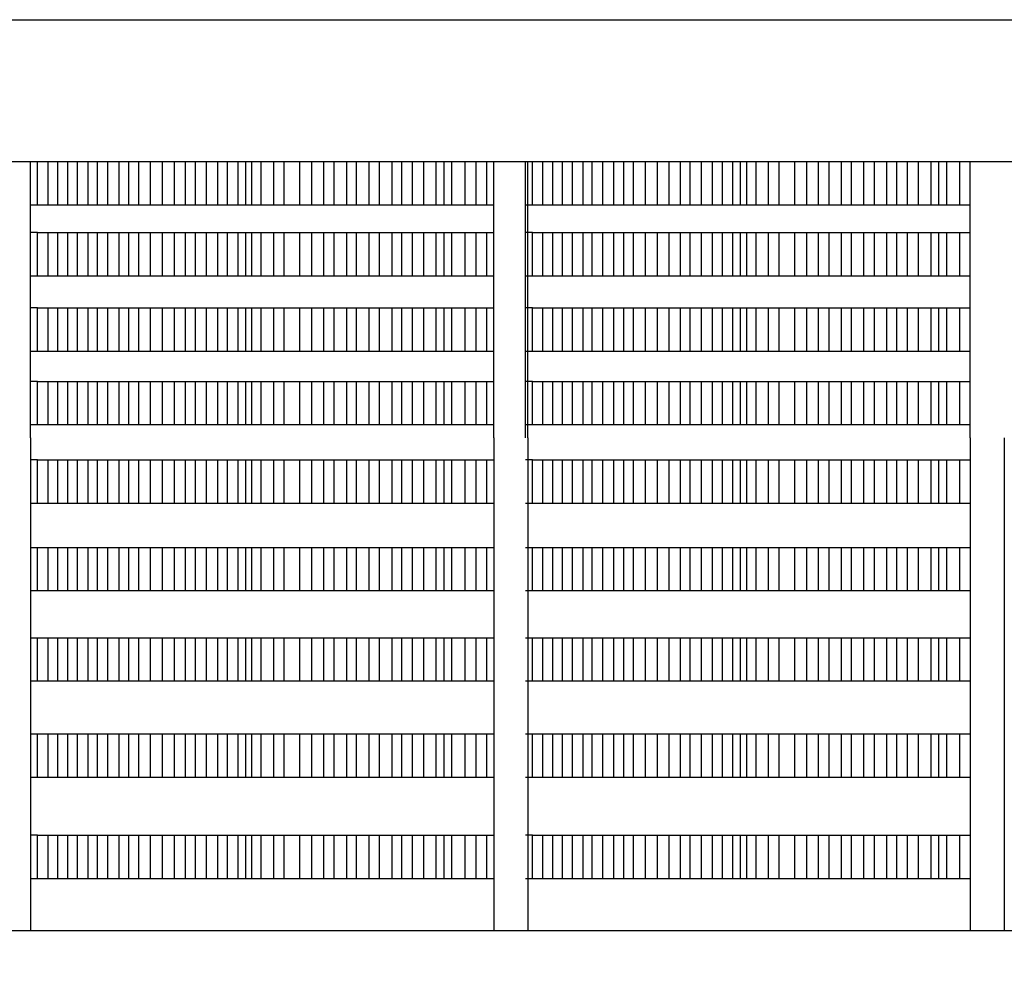
# Model space of a CAD drawing. Units: inches. Extents: x -117 to 121, y -77 to 40.
# Tile 33 of 45: x 34.28 to 45.7, y 10.29 to 21.31. Entities that reach past the tile are written whole.
import ezdxf

# ---------------------------------------------------------------- set-up
doc = ezdxf.new("R2010")
doc.units = ezdxf.units.IN
doc.header["$MEASUREMENT"] = 0
doc.layers.add('A-ANNO-DIMS', color=2, linetype='Continuous', lineweight=18)
doc.layers.add('A-ELEV', color=7, linetype='Continuous', lineweight=25)
doc.styles.get("Standard").update_dxf_attribs({"font": 'arial.ttf'})
doc.dimstyles.get("Standard").update_dxf_attribs({"dimtxt": 0.18, "dimasz": 0.18, "dimexe": 0.18, "dimexo": 0.0625, "dimgap": 0.09, "dimtad": 0, "dimtih": 1, "dimtoh": 1, "dimdec": 4, "dimzin": 0, "dimdsep": 46, "dimtxsty": 'Standard', "dimcen": 0.09, "dimadec": 0, "dimazin": 0, "dimtfac": 1, "dimtdec": 4, "dimtofl": 0, "dimtmove": 0, "dimatfit": 3, "dimfxl": 1, "dimtolj": 1, "dimtzin": 0, "dimarcsym": 0})

# ---------------------------------------------------------------- blocks, each defined once
blk = doc.blocks.new('*D53')
at = {"layer": 'A-ANNO-DIMS', "color": 0, "lineweight": -2, "transparency": 16777216}
for p, q in [((51.69, 10.9), (51.69, -77.193)), ((27.974, 10.841), (27.974, -77.193)), ((28.154, -77.013), (39.367, -77.013)), ((51.51, -77.013), (40.297, -77.013))]:
    blk.add_line(p, q, dxfattribs=at)
at = {"layer": 'A-ANNO-DIMS', "color": 0, "transparency": 16777216}
for points in [[(28.154, -76.983), (28.154, -77.043), (27.974, -77.013)], [(51.51, -76.983), (51.51, -77.043), (51.69, -77.013)]]:
    blk.add_solid(points, dxfattribs=at)
at = {"layer": 'Defpoints', "color": 0, "transparency": 16777216}
for p in [(51.69, 10.962), (27.974, 10.903), (51.69, -77.013)]:
    blk.add_point(p, dxfattribs=at)
at = {"layer": 'A-ANNO-DIMS', "color": 0, "transparency": 16777216, "insert": (39.832, -77.013), "char_height": 0.18, "attachment_point": 5}
blk.add_mtext('\\A1;23.716', dxfattribs=at)

msp = doc.modelspace()

# ---------------------------------------------------------------- linework, layer by layer
at = {"layer": 'A-ELEV'}
for p, q in [((32.0351, 21.3104), (70.6115, 21.3104)), ((27.8529, 19.6653), (51.6089, 19.6653)), ((34.4079, 16.4655), (34.4079, 19.6653)), ((34.4891, 19.1644), (34.4891, 19.6653)), ((34.6111, 19.1644), (34.6111, 19.6653)), ((34.7255, 19.1644), (34.7255, 19.6653)), ((34.8399, 19.1644), (34.8399, 19.6653)), ((34.9543, 19.1644), (34.9543, 19.6653)), ((35.0763, 19.1644), (35.0763, 19.6653)), ((35.1831, 19.1644), (35.1831, 19.6653)), ((35.3051, 19.1644), (35.3051, 19.6653)), ((35.4347, 19.1644), (35.4347, 19.6653)), ((35.5491, 19.1644), (35.5491, 19.6653)), ((35.6635, 19.1644), (35.6635, 19.6653)), ((35.8008, 19.1644), (35.8008, 19.6653)), ((35.9381, 19.1644), (35.9381, 19.6653)), ((36.0753, 19.1644), (36.0753, 19.6653)), ((36.205, 19.1644), (36.205, 19.6653)), ((36.3194, 19.1644), (36.3194, 19.6653)), ((36.449, 19.1644), (36.449, 19.6653)), ((36.5787, 19.1644), (36.5787, 19.6653)), ((36.6931, 19.1644), (36.6931, 19.6653)), ((36.8151, 19.1644), (36.8151, 19.6653)), ((36.9029, 19.1644), (36.9029, 19.6562)), ((36.9752, 19.1644), (36.9752, 19.6653)), ((37.082, 19.1644), (37.082, 19.6653)), ((37.2269, 19.1644), (37.2269, 19.6653)), ((37.3489, 19.1644), (37.3489, 19.6653)), ((37.5319, 19.1644), (37.5319, 19.6653)), ((37.6692, 19.1644), (37.6692, 19.6653)), ((37.8065, 19.1644), (37.8065, 19.6653)), ((37.9285, 19.1644), (37.9285, 19.6653)), ((38.0734, 19.1644), (38.0734, 19.6653)), ((38.1878, 19.1644), (38.1878, 19.6653)), ((38.3327, 19.1644), (38.3327, 19.6653)), ((38.4547, 19.1644), (38.4547, 19.6653)), ((38.5996, 19.1644), (38.5996, 19.6653)), ((38.714, 19.1644), (38.714, 19.6653)), ((38.836, 19.1644), (38.836, 19.6653)), ((38.9657, 19.1644), (38.9657, 19.6653)), ((39.1106, 19.1644), (39.1106, 19.6653)), ((39.2021, 19.1644), (39.2021, 19.6653)), ((39.2936, 19.1644), (39.2936, 19.6653)), ((39.4461, 19.1644), (39.4461, 19.6653)), ((39.5758, 19.1644), (39.5758, 19.6653)), ((39.6978, 19.1644), (39.6978, 19.6653)), ((39.7801, 16.4655), (39.7801, 19.6653)), ((40.1443, 16.4655), (40.1443, 19.6653)), ((40.1744, 16.4655), (40.1744, 19.6653)), ((40.2255, 19.1644), (40.2255, 19.6653)), ((40.3475, 19.1644), (40.3475, 19.6653)), ((40.4619, 19.1644), (40.4619, 19.6653)), ((40.5763, 19.1644), (40.5763, 19.6653)), ((40.6907, 19.1644), (40.6907, 19.6653)), ((40.8127, 19.1644), (40.8127, 19.6653)), ((40.9194, 19.1644), (40.9194, 19.6653)), ((41.0415, 19.1644), (41.0415, 19.6653)), ((41.1711, 19.1644), (41.1711, 19.6653)), ((41.2855, 19.1644), (41.2855, 19.6653)), ((41.3999, 19.1644), (41.3999, 19.6653)), ((41.5372, 19.1644), (41.5372, 19.6653)), ((41.6744, 19.1644), (41.6744, 19.6653)), ((41.8117, 19.1644), (41.8117, 19.6653)), ((41.9414, 19.1644), (41.9414, 19.6653)), ((42.0557, 19.1644), (42.0557, 19.6653)), ((42.1854, 19.1644), (42.1854, 19.6653)), ((42.315, 19.1644), (42.315, 19.6653)), ((42.4294, 19.1644), (42.4294, 19.6653)), ((42.5514, 19.1644), (42.5514, 19.6653)), ((42.6392, 19.1644), (42.6392, 19.6562)), ((42.7116, 19.1644), (42.7116, 19.6653)), ((42.8184, 19.1644), (42.8184, 19.6653)), ((42.9633, 19.1644), (42.9633, 19.6653)), ((43.0853, 19.1644), (43.0853, 19.6653)), ((43.2683, 19.1644), (43.2683, 19.6653)), ((43.4056, 19.1644), (43.4056, 19.6653)), ((43.5429, 19.1644), (43.5429, 19.6653)), ((43.6649, 19.1644), (43.6649, 19.6653)), ((43.8098, 19.1644), (43.8098, 19.6653)), ((43.9242, 19.1644), (43.9242, 19.6653)), ((44.0691, 19.1644), (44.0691, 19.6653)), ((44.1911, 19.1644), (44.1911, 19.6653)), ((44.336, 19.1644), (44.336, 19.6653)), ((44.4504, 19.1644), (44.4504, 19.6653)), ((44.5724, 19.1644), (44.5724, 19.6653)), ((44.702, 19.1644), (44.702, 19.6653)), ((44.8469, 19.1644), (44.8469, 19.6653)), ((44.9384, 19.1644), (44.9384, 19.6653)), ((45.03, 19.1644), (45.03, 19.6653)), ((45.1825, 19.1644), (45.1825, 19.6653)), ((45.3002, 16.4655), (45.3002, 19.6653)), ((34.4079, 19.1644), (39.7801, 19.1644)), ((40.1443, 19.1644), (45.3002, 19.1644)), ((34.4891, 18.8424), (34.4079, 18.8424)), ((34.4891, 18.3415), (34.4891, 18.8424)), ((34.4891, 18.8424), (39.7801, 18.8424)), ((34.6111, 18.3415), (34.6111, 18.8424)), ((34.7255, 18.3415), (34.7255, 18.8424)), ((34.8399, 18.3415), (34.8399, 18.8424)), ((34.9543, 18.3415), (34.9543, 18.8424)), ((35.0763, 18.3415), (35.0763, 18.8424)), ((35.1831, 18.3415), (35.1831, 18.8424)), ((35.3051, 18.3415), (35.3051, 18.8424)), ((35.4347, 18.3415), (35.4347, 18.8424)), ((35.5491, 18.3415), (35.5491, 18.8424)), ((35.6635, 18.3415), (35.6635, 18.8424)), ((35.8008, 18.3415), (35.8008, 18.8424)), ((35.9381, 18.3415), (35.9381, 18.8424)), ((36.0753, 18.3415), (36.0753, 18.8424)), ((36.205, 18.3415), (36.205, 18.8424)), ((36.3194, 18.3415), (36.3194, 18.8424)), ((36.449, 18.3415), (36.449, 18.8424)), ((36.5787, 18.3415), (36.5787, 18.8424)), ((36.6931, 18.3415), (36.6931, 18.8424)), ((36.8151, 18.3415), (36.8151, 18.8424)), ((36.9029, 18.3415), (36.9029, 18.8333)), ((36.9752, 18.3415), (36.9752, 18.8424)), ((37.082, 18.3415), (37.082, 18.8424)), ((37.2269, 18.3415), (37.2269, 18.8424)), ((37.3489, 18.3415), (37.3489, 18.8424)), ((37.5319, 18.3415), (37.5319, 18.8424)), ((37.6692, 18.3415), (37.6692, 18.8424)), ((37.8065, 18.3415), (37.8065, 18.8424)), ((37.9285, 18.3415), (37.9285, 18.8424)), ((38.0734, 18.3415), (38.0734, 18.8424)), ((38.1878, 18.3415), (38.1878, 18.8424)), ((38.3327, 18.3415), (38.3327, 18.8424)), ((38.4547, 18.3415), (38.4547, 18.8424)), ((38.5996, 18.3415), (38.5996, 18.8424)), ((38.714, 18.3415), (38.714, 18.8424)), ((38.836, 18.3415), (38.836, 18.8424)), ((38.9657, 18.3415), (38.9657, 18.8424)), ((39.1106, 18.3415), (39.1106, 18.8424)), ((39.2021, 18.3415), (39.2021, 18.8424)), ((39.2936, 18.3415), (39.2936, 18.8424)), ((39.4461, 18.3415), (39.4461, 18.8424)), ((39.5758, 18.3415), (39.5758, 18.8424)), ((39.6978, 18.3415), (39.6978, 18.8424)), ((40.2255, 18.8424), (40.1443, 18.8424)), ((40.2255, 18.3415), (40.2255, 18.8424)), ((40.2255, 18.8424), (45.3002, 18.8424)), ((40.3475, 18.3415), (40.3475, 18.8424)), ((40.4619, 18.3415), (40.4619, 18.8424)), ((40.5763, 18.3415), (40.5763, 18.8424)), ((40.6907, 18.3415), (40.6907, 18.8424)), ((40.8127, 18.3415), (40.8127, 18.8424)), ((40.9194, 18.3415), (40.9194, 18.8424)), ((41.0415, 18.3415), (41.0415, 18.8424)), ((41.1711, 18.3415), (41.1711, 18.8424)), ((41.2855, 18.3415), (41.2855, 18.8424)), ((41.3999, 18.3415), (41.3999, 18.8424)), ((41.5372, 18.3415), (41.5372, 18.8424)), ((41.6744, 18.3415), (41.6744, 18.8424)), ((41.8117, 18.3415), (41.8117, 18.8424)), ((41.9414, 18.3415), (41.9414, 18.8424)), ((42.0557, 18.3415), (42.0557, 18.8424)), ((42.1854, 18.3415), (42.1854, 18.8424)), ((42.315, 18.3415), (42.315, 18.8424)), ((42.4294, 18.3415), (42.4294, 18.8424)), ((42.5514, 18.3415), (42.5514, 18.8424)), ((42.6392, 18.3415), (42.6392, 18.8333)), ((42.7116, 18.3415), (42.7116, 18.8424)), ((42.8184, 18.3415), (42.8184, 18.8424)), ((42.9633, 18.3415), (42.9633, 18.8424)), ((43.0853, 18.3415), (43.0853, 18.8424)), ((43.2683, 18.3415), (43.2683, 18.8424)), ((43.4056, 18.3415), (43.4056, 18.8424)), ((43.5429, 18.3415), (43.5429, 18.8424)), ((43.6649, 18.3415), (43.6649, 18.8424)), ((43.8098, 18.3415), (43.8098, 18.8424)), ((43.9242, 18.3415), (43.9242, 18.8424)), ((44.0691, 18.3415), (44.0691, 18.8424)), ((44.1911, 18.3415), (44.1911, 18.8424)), ((44.336, 18.3415), (44.336, 18.8424)), ((44.4504, 18.3415), (44.4504, 18.8424)), ((44.5724, 18.3415), (44.5724, 18.8424)), ((44.702, 18.3415), (44.702, 18.8424)), ((44.8469, 18.3415), (44.8469, 18.8424)), ((44.9384, 18.3415), (44.9384, 18.8424)), ((45.03, 18.3415), (45.03, 18.8424)), ((45.1825, 18.3415), (45.1825, 18.8424)), ((34.4079, 18.3415), (39.7801, 18.3415)), ((40.1443, 18.3415), (45.3002, 18.3415)), ((34.4891, 17.9696), (34.4079, 17.9696)), ((34.4891, 17.4687), (34.4891, 17.9696)), ((34.4891, 17.9696), (39.7801, 17.9696)), ((34.6111, 17.4687), (34.6111, 17.9696)), ((34.7255, 17.4687), (34.7255, 17.9696)), ((34.8399, 17.4687), (34.8399, 17.9696)), ((34.9543, 17.4687), (34.9543, 17.9696)), ((35.0763, 17.4687), (35.0763, 17.9696)), ((35.1831, 17.4687), (35.1831, 17.9696)), ((35.3051, 17.4687), (35.3051, 17.9696)), ((35.4347, 17.4687), (35.4347, 17.9696)), ((35.5491, 17.4687), (35.5491, 17.9696)), ((35.6635, 17.4687), (35.6635, 17.9696)), ((35.8008, 17.4687), (35.8008, 17.9696)), ((35.9381, 17.4687), (35.9381, 17.9696)), ((36.0753, 17.4687), (36.0753, 17.9696)), ((36.205, 17.4687), (36.205, 17.9696)), ((36.3194, 17.4687), (36.3194, 17.9696)), ((36.449, 17.4687), (36.449, 17.9696)), ((36.5787, 17.4687), (36.5787, 17.9696)), ((36.6931, 17.4687), (36.6931, 17.9696)), ((36.8151, 17.4687), (36.8151, 17.9696)), ((36.9029, 17.4687), (36.9029, 17.9605)), ((36.9752, 17.4687), (36.9752, 17.9696)), ((37.082, 17.4687), (37.082, 17.9696)), ((37.2269, 17.4687), (37.2269, 17.9696)), ((37.3489, 17.4687), (37.3489, 17.9696)), ((37.5319, 17.4687), (37.5319, 17.9696)), ((37.6692, 17.4687), (37.6692, 17.9696)), ((37.8065, 17.4687), (37.8065, 17.9696)), ((37.9285, 17.4687), (37.9285, 17.9696)), ((38.0734, 17.4687), (38.0734, 17.9696)), ((38.1878, 17.4687), (38.1878, 17.9696)), ((38.3327, 17.4687), (38.3327, 17.9696)), ((38.4547, 17.4687), (38.4547, 17.9696)), ((38.5996, 17.4687), (38.5996, 17.9696)), ((38.714, 17.4687), (38.714, 17.9696)), ((38.836, 17.4687), (38.836, 17.9696)), ((38.9657, 17.4687), (38.9657, 17.9696)), ((39.1106, 17.4687), (39.1106, 17.9696)), ((39.2021, 17.4687), (39.2021, 17.9696)), ((39.2936, 17.4687), (39.2936, 17.9696)), ((39.4461, 17.4687), (39.4461, 17.9696)), ((39.5758, 17.4687), (39.5758, 17.9696)), ((39.6978, 17.4687), (39.6978, 17.9696)), ((40.2255, 17.9696), (40.1443, 17.9696)), ((40.2255, 17.4687), (40.2255, 17.9696)), ((40.2255, 17.9696), (45.3002, 17.9696)), ((40.3475, 17.4687), (40.3475, 17.9696)), ((40.4619, 17.4687), (40.4619, 17.9696)), ((40.5763, 17.4687), (40.5763, 17.9696)), ((40.6907, 17.4687), (40.6907, 17.9696)), ((40.8127, 17.4687), (40.8127, 17.9696)), ((40.9194, 17.4687), (40.9194, 17.9696)), ((41.0415, 17.4687), (41.0415, 17.9696)), ((41.1711, 17.4687), (41.1711, 17.9696)), ((41.2855, 17.4687), (41.2855, 17.9696)), ((41.3999, 17.4687), (41.3999, 17.9696)), ((41.5372, 17.4687), (41.5372, 17.9696)), ((41.6744, 17.4687), (41.6744, 17.9696)), ((41.8117, 17.4687), (41.8117, 17.9696)), ((41.9414, 17.4687), (41.9414, 17.9696)), ((42.0557, 17.4687), (42.0557, 17.9696)), ((42.1854, 17.4687), (42.1854, 17.9696)), ((42.315, 17.4687), (42.315, 17.9696)), ((42.4294, 17.4687), (42.4294, 17.9696)), ((42.5514, 17.4687), (42.5514, 17.9696)), ((42.6392, 17.4687), (42.6392, 17.9605)), ((42.7116, 17.4687), (42.7116, 17.9696)), ((42.8184, 17.4687), (42.8184, 17.9696)), ((42.9633, 17.4687), (42.9633, 17.9696)), ((43.0853, 17.4687), (43.0853, 17.9696)), ((43.2683, 17.4687), (43.2683, 17.9696)), ((43.4056, 17.4687), (43.4056, 17.9696)), ((43.5429, 17.4687), (43.5429, 17.9696)), ((43.6649, 17.4687), (43.6649, 17.9696)), ((43.8098, 17.4687), (43.8098, 17.9696)), ((43.9242, 17.4687), (43.9242, 17.9696)), ((44.0691, 17.4687), (44.0691, 17.9696)), ((44.1911, 17.4687), (44.1911, 17.9696)), ((44.336, 17.4687), (44.336, 17.9696)), ((44.4504, 17.4687), (44.4504, 17.9696)), ((44.5724, 17.4687), (44.5724, 17.9696)), ((44.702, 17.4687), (44.702, 17.9696)), ((44.8469, 17.4687), (44.8469, 17.9696)), ((44.9384, 17.4687), (44.9384, 17.9696)), ((45.03, 17.4687), (45.03, 17.9696)), ((45.1825, 17.4687), (45.1825, 17.9696)), ((34.4079, 17.4687), (39.7801, 17.4687)), ((40.1443, 17.4687), (45.3002, 17.4687)), ((34.4891, 17.1187), (34.4079, 17.1187)), ((34.4891, 16.6179), (34.4891, 17.1187)), ((34.4891, 17.1187), (39.7801, 17.1187)), ((34.6111, 16.6179), (34.6111, 17.1187)), ((34.7255, 16.6179), (34.7255, 17.1187)), ((34.8399, 16.6179), (34.8399, 17.1187)), ((34.9543, 16.6179), (34.9543, 17.1187)), ((35.0763, 16.6179), (35.0763, 17.1187)), ((35.1831, 16.6179), (35.1831, 17.1187)), ((35.3051, 16.6179), (35.3051, 17.1187)), ((35.4347, 16.6179), (35.4347, 17.1187)), ((35.5491, 16.6179), (35.5491, 17.1187)), ((35.6635, 16.6179), (35.6635, 17.1187)), ((35.8008, 16.6179), (35.8008, 17.1187)), ((35.9381, 16.6179), (35.9381, 17.1187)), ((36.0753, 16.6179), (36.0753, 17.1187)), ((36.205, 16.6179), (36.205, 17.1187)), ((36.3194, 16.6179), (36.3194, 17.1187)), ((36.449, 16.6179), (36.449, 17.1187)), ((36.5787, 16.6179), (36.5787, 17.1187)), ((36.6931, 16.6179), (36.6931, 17.1187)), ((36.8151, 16.6179), (36.8151, 17.1187)), ((36.9029, 16.6179), (36.9029, 17.1097)), ((36.9752, 16.6179), (36.9752, 17.1187)), ((37.082, 16.6179), (37.082, 17.1187)), ((37.2269, 16.6179), (37.2269, 17.1187)), ((37.3489, 16.6179), (37.3489, 17.1187)), ((37.5319, 16.6179), (37.5319, 17.1187)), ((37.6692, 16.6179), (37.6692, 17.1187)), ((37.8065, 16.6179), (37.8065, 17.1187)), ((37.9285, 16.6179), (37.9285, 17.1187)), ((38.0734, 16.6179), (38.0734, 17.1187)), ((38.1878, 16.6179), (38.1878, 17.1187)), ((38.3327, 16.6179), (38.3327, 17.1187)), ((38.4547, 16.6179), (38.4547, 17.1187)), ((38.5996, 16.6179), (38.5996, 17.1187)), ((38.714, 16.6179), (38.714, 17.1187)), ((38.836, 16.6179), (38.836, 17.1187)), ((38.9657, 16.6179), (38.9657, 17.1187)), ((39.1106, 16.6179), (39.1106, 17.1187)), ((39.2021, 16.6179), (39.2021, 17.1187)), ((39.2936, 16.6179), (39.2936, 17.1187)), ((39.4461, 16.6179), (39.4461, 17.1187)), ((39.5758, 16.6179), (39.5758, 17.1187)), ((39.6978, 16.6179), (39.6978, 17.1187)), ((40.2255, 17.1187), (40.1443, 17.1187)), ((40.2255, 16.6179), (40.2255, 17.1187)), ((40.2255, 17.1187), (45.3002, 17.1187)), ((40.3475, 16.6179), (40.3475, 17.1187)), ((40.4619, 16.6179), (40.4619, 17.1187)), ((40.5763, 16.6179), (40.5763, 17.1187)), ((40.6907, 16.6179), (40.6907, 17.1187)), ((40.8127, 16.6179), (40.8127, 17.1187)), ((40.9194, 16.6179), (40.9194, 17.1187)), ((41.0415, 16.6179), (41.0415, 17.1187)), ((41.1711, 16.6179), (41.1711, 17.1187)), ((41.2855, 16.6179), (41.2855, 17.1187)), ((41.3999, 16.6179), (41.3999, 17.1187)), ((41.5372, 16.6179), (41.5372, 17.1187)), ((41.6744, 16.6179), (41.6744, 17.1187)), ((41.8117, 16.6179), (41.8117, 17.1187)), ((41.9414, 16.6179), (41.9414, 17.1187)), ((42.0557, 16.6179), (42.0557, 17.1187)), ((42.1854, 16.6179), (42.1854, 17.1187)), ((42.315, 16.6179), (42.315, 17.1187)), ((42.4294, 16.6179), (42.4294, 17.1187)), ((42.5514, 16.6179), (42.5514, 17.1187)), ((42.6392, 16.6179), (42.6392, 17.1097)), ((42.7116, 16.6179), (42.7116, 17.1187)), ((42.8184, 16.6179), (42.8184, 17.1187)), ((42.9633, 16.6179), (42.9633, 17.1187)), ((43.0853, 16.6179), (43.0853, 17.1187)), ((43.2683, 16.6179), (43.2683, 17.1187)), ((43.4056, 16.6179), (43.4056, 17.1187)), ((43.5429, 16.6179), (43.5429, 17.1187)), ((43.6649, 16.6179), (43.6649, 17.1187)), ((43.8098, 16.6179), (43.8098, 17.1187)), ((43.9242, 16.6179), (43.9242, 17.1187)), ((44.0691, 16.6179), (44.0691, 17.1187)), ((44.1911, 16.6179), (44.1911, 17.1187)), ((44.336, 16.6179), (44.336, 17.1187)), ((44.4504, 16.6179), (44.4504, 17.1187)), ((44.5724, 16.6179), (44.5724, 17.1187)), ((44.702, 16.6179), (44.702, 17.1187)), ((44.8469, 16.6179), (44.8469, 17.1187)), ((44.9384, 16.6179), (44.9384, 17.1187)), ((45.03, 16.6179), (45.03, 17.1187)), ((45.1825, 16.6179), (45.1825, 17.1187)), ((34.4079, 16.6179), (39.7801, 16.6179)), ((40.1443, 16.6179), (45.3002, 16.6179)), ((34.4079, 16.4655), (34.4079, 10.755)), ((39.7801, 16.4655), (39.7801, 10.755)), ((40.1744, 16.4655), (40.1744, 10.755)), ((45.3002, 16.4655), (45.3002, 10.755)), ((45.6945, 16.4655), (45.6945, 10.755)), ((34.4891, 16.2085), (34.4079, 16.2085)), ((34.4891, 15.7077), (34.4891, 16.2085)), ((34.4891, 16.2085), (39.7801, 16.2085)), ((34.6111, 15.7077), (34.6111, 16.2085)), ((34.7255, 15.7077), (34.7255, 16.2085)), ((34.8399, 15.7077), (34.8399, 16.2085)), ((34.9543, 15.7077), (34.9543, 16.2085)), ((35.0763, 15.7077), (35.0763, 16.2085)), ((35.1831, 15.7077), (35.1831, 16.2085)), ((35.3051, 15.7077), (35.3051, 16.2085)), ((35.4347, 15.7077), (35.4347, 16.2085)), ((35.5491, 15.7077), (35.5491, 16.2085)), ((35.6635, 15.7077), (35.6635, 16.2085)), ((35.8008, 15.7077), (35.8008, 16.2085)), ((35.9381, 15.7077), (35.9381, 16.2085)), ((36.0753, 15.7077), (36.0753, 16.2085)), ((36.205, 15.7077), (36.205, 16.2085)), ((36.3194, 15.7077), (36.3194, 16.2085)), ((36.449, 15.7077), (36.449, 16.2085)), ((36.5787, 15.7077), (36.5787, 16.2085)), ((36.6931, 15.7077), (36.6931, 16.2085)), ((36.8151, 15.7077), (36.8151, 16.2085)), ((36.9752, 15.7077), (36.9752, 16.2085)), ((37.082, 15.7077), (37.082, 16.2085)), ((37.2269, 15.7077), (37.2269, 16.2085)), ((37.3489, 15.7077), (37.3489, 16.2085)), ((37.5319, 15.7077), (37.5319, 16.2085)), ((37.6692, 15.7077), (37.6692, 16.2085)), ((37.8065, 15.7077), (37.8065, 16.2085)), ((37.9285, 15.7077), (37.9285, 16.2085)), ((38.0734, 15.7077), (38.0734, 16.2085)), ((38.1878, 15.7077), (38.1878, 16.2085)), ((38.3327, 15.7077), (38.3327, 16.2085)), ((38.4547, 15.7077), (38.4547, 16.2085)), ((38.5996, 15.7077), (38.5996, 16.2085)), ((38.714, 15.7077), (38.714, 16.2085)), ((38.836, 15.7077), (38.836, 16.2085)), ((38.9657, 15.7077), (38.9657, 16.2085)), ((39.1106, 15.7077), (39.1106, 16.2085)), ((39.2021, 15.7077), (39.2021, 16.2085)), ((39.2936, 15.7077), (39.2936, 16.2085)), ((39.4461, 15.7077), (39.4461, 16.2085)), ((39.5758, 15.7077), (39.5758, 16.2085)), ((39.6978, 15.7077), (39.6978, 16.2085)), ((40.2255, 16.2085), (40.1443, 16.2085)), ((40.2255, 15.7077), (40.2255, 16.2085)), ((40.2255, 16.2085), (45.3002, 16.2085)), ((40.3475, 15.7077), (40.3475, 16.2085)), ((40.4619, 15.7077), (40.4619, 16.2085)), ((40.5763, 15.7077), (40.5763, 16.2085)), ((40.6907, 15.7077), (40.6907, 16.2085)), ((40.8127, 15.7077), (40.8127, 16.2085)), ((40.9194, 15.7077), (40.9194, 16.2085)), ((41.0415, 15.7077), (41.0415, 16.2085)), ((41.1711, 15.7077), (41.1711, 16.2085)), ((41.2855, 15.7077), (41.2855, 16.2085)), ((41.3999, 15.7077), (41.3999, 16.2085)), ((41.5372, 15.7077), (41.5372, 16.2085)), ((41.6744, 15.7077), (41.6744, 16.2085)), ((41.8117, 15.7077), (41.8117, 16.2085)), ((41.9414, 15.7077), (41.9414, 16.2085)), ((42.0557, 15.7077), (42.0557, 16.2085)), ((42.1854, 15.7077), (42.1854, 16.2085)), ((42.315, 15.7077), (42.315, 16.2085)), ((42.4294, 15.7077), (42.4294, 16.2085)), ((42.5514, 15.7077), (42.5514, 16.2085)), ((42.7116, 15.7077), (42.7116, 16.2085)), ((42.8184, 15.7077), (42.8184, 16.2085)), ((42.9633, 15.7077), (42.9633, 16.2085)), ((43.0853, 15.7077), (43.0853, 16.2085)), ((43.2683, 15.7077), (43.2683, 16.2085)), ((43.4056, 15.7077), (43.4056, 16.2085)), ((43.5429, 15.7077), (43.5429, 16.2085)), ((43.6649, 15.7077), (43.6649, 16.2085)), ((43.8098, 15.7077), (43.8098, 16.2085)), ((43.9242, 15.7077), (43.9242, 16.2085)), ((44.0691, 15.7077), (44.0691, 16.2085)), ((44.1911, 15.7077), (44.1911, 16.2085)), ((44.336, 15.7077), (44.336, 16.2085)), ((44.4504, 15.7077), (44.4504, 16.2085)), ((44.5724, 15.7077), (44.5724, 16.2085)), ((44.702, 15.7077), (44.702, 16.2085)), ((44.8469, 15.7077), (44.8469, 16.2085)), ((44.9384, 15.7077), (44.9384, 16.2085)), ((45.03, 15.7077), (45.03, 16.2085)), ((45.1825, 15.7077), (45.1825, 16.2085)), ((36.9029, 15.7077), (36.9029, 16.1995)), ((42.6392, 15.7077), (42.6392, 16.1995)), ((34.4079, 15.7077), (39.7801, 15.7077)), ((40.1443, 15.7077), (45.3002, 15.7077)), ((34.4079, 15.1944), (39.7801, 15.1944)), ((34.4891, 14.6936), (34.4891, 15.1944)), ((34.6111, 14.6936), (34.6111, 15.1944)), ((34.7255, 14.6936), (34.7255, 15.1944)), ((34.8399, 14.6936), (34.8399, 15.1944)), ((34.9543, 14.6936), (34.9543, 15.1944)), ((35.0763, 14.6936), (35.0763, 15.1944)), ((35.1831, 14.6936), (35.1831, 15.1944)), ((35.3051, 14.6936), (35.3051, 15.1944)), ((35.4347, 14.6936), (35.4347, 15.1944)), ((35.5491, 14.6936), (35.5491, 15.1944)), ((35.6635, 14.6936), (35.6635, 15.1944)), ((35.8008, 14.6936), (35.8008, 15.1944)), ((35.9381, 14.6936), (35.9381, 15.1944)), ((36.0753, 14.6936), (36.0753, 15.1944)), ((36.205, 14.6936), (36.205, 15.1944)), ((36.3194, 14.6936), (36.3194, 15.1944)), ((36.449, 14.6936), (36.449, 15.1944)), ((36.5787, 14.6936), (36.5787, 15.1944)), ((36.6931, 14.6936), (36.6931, 15.1944)), ((36.8151, 14.6936), (36.8151, 15.1944)), ((36.9029, 14.6936), (36.9029, 15.1854)), ((36.9752, 14.6936), (36.9752, 15.1944)), ((37.082, 14.6936), (37.082, 15.1944)), ((37.2269, 14.6936), (37.2269, 15.1944)), ((37.3489, 14.6936), (37.3489, 15.1944)), ((37.5319, 14.6936), (37.5319, 15.1944)), ((37.6692, 14.6936), (37.6692, 15.1944)), ((37.8065, 14.6936), (37.8065, 15.1944)), ((37.9285, 14.6936), (37.9285, 15.1944)), ((38.0734, 14.6936), (38.0734, 15.1944)), ((38.1878, 14.6936), (38.1878, 15.1944)), ((38.3327, 14.6936), (38.3327, 15.1944)), ((38.4547, 14.6936), (38.4547, 15.1944)), ((38.5996, 14.6936), (38.5996, 15.1944)), ((38.714, 14.6936), (38.714, 15.1944)), ((38.836, 14.6936), (38.836, 15.1944)), ((38.9657, 14.6936), (38.9657, 15.1944)), ((39.1106, 14.6936), (39.1106, 15.1944)), ((39.2021, 14.6936), (39.2021, 15.1944)), ((39.2936, 14.6936), (39.2936, 15.1944)), ((39.4461, 14.6936), (39.4461, 15.1944)), ((39.5758, 14.6936), (39.5758, 15.1944)), ((39.6978, 14.6936), (39.6978, 15.1944)), ((40.1443, 15.1944), (45.3002, 15.1944)), ((40.2255, 14.6936), (40.2255, 15.1944)), ((40.3475, 14.6936), (40.3475, 15.1944)), ((40.4619, 14.6936), (40.4619, 15.1944)), ((40.5763, 14.6936), (40.5763, 15.1944)), ((40.6907, 14.6936), (40.6907, 15.1944)), ((40.8127, 14.6936), (40.8127, 15.1944)), ((40.9194, 14.6936), (40.9194, 15.1944)), ((41.0415, 14.6936), (41.0415, 15.1944)), ((41.1711, 14.6936), (41.1711, 15.1944)), ((41.2855, 14.6936), (41.2855, 15.1944)), ((41.3999, 14.6936), (41.3999, 15.1944)), ((41.5372, 14.6936), (41.5372, 15.1944)), ((41.6744, 14.6936), (41.6744, 15.1944)), ((41.8117, 14.6936), (41.8117, 15.1944)), ((41.9414, 14.6936), (41.9414, 15.1944)), ((42.0557, 14.6936), (42.0557, 15.1944)), ((42.1854, 14.6936), (42.1854, 15.1944)), ((42.315, 14.6936), (42.315, 15.1944)), ((42.4294, 14.6936), (42.4294, 15.1944)), ((42.5514, 14.6936), (42.5514, 15.1944)), ((42.6392, 14.6936), (42.6392, 15.1854)), ((42.7116, 14.6936), (42.7116, 15.1944)), ((42.8184, 14.6936), (42.8184, 15.1944)), ((42.9633, 14.6936), (42.9633, 15.1944)), ((43.0853, 14.6936), (43.0853, 15.1944)), ((43.2683, 14.6936), (43.2683, 15.1944)), ((43.4056, 14.6936), (43.4056, 15.1944)), ((43.5429, 14.6936), (43.5429, 15.1944)), ((43.6649, 14.6936), (43.6649, 15.1944)), ((43.8098, 14.6936), (43.8098, 15.1944)), ((43.9242, 14.6936), (43.9242, 15.1944)), ((44.0691, 14.6936), (44.0691, 15.1944)), ((44.1911, 14.6936), (44.1911, 15.1944)), ((44.336, 14.6936), (44.336, 15.1944)), ((44.4504, 14.6936), (44.4504, 15.1944)), ((44.5724, 14.6936), (44.5724, 15.1944)), ((44.702, 14.6936), (44.702, 15.1944)), ((44.8469, 14.6936), (44.8469, 15.1944)), ((44.9384, 14.6936), (44.9384, 15.1944)), ((45.03, 14.6936), (45.03, 15.1944)), ((45.1825, 14.6936), (45.1825, 15.1944)), ((34.4079, 14.6936), (39.7801, 14.6936)), ((40.1443, 14.6936), (45.3002, 14.6936)), ((34.4079, 14.1471), (39.7801, 14.1471)), ((34.4891, 13.6462), (34.4891, 14.1471)), ((34.6111, 13.6462), (34.6111, 14.1471)), ((34.7255, 13.6462), (34.7255, 14.1471)), ((34.8399, 13.6462), (34.8399, 14.1471)), ((34.9543, 13.6462), (34.9543, 14.1471)), ((35.0763, 13.6462), (35.0763, 14.1471)), ((35.1831, 13.6462), (35.1831, 14.1471)), ((35.3051, 13.6462), (35.3051, 14.1471)), ((35.4347, 13.6462), (35.4347, 14.1471)), ((35.5491, 13.6462), (35.5491, 14.1471)), ((35.6635, 13.6462), (35.6635, 14.1471)), ((35.8008, 13.6462), (35.8008, 14.1471)), ((35.9381, 13.6462), (35.9381, 14.1471)), ((36.0753, 13.6462), (36.0753, 14.1471)), ((36.205, 13.6462), (36.205, 14.1471)), ((36.3194, 13.6462), (36.3194, 14.1471)), ((36.449, 13.6462), (36.449, 14.1471)), ((36.5787, 13.6462), (36.5787, 14.1471)), ((36.6931, 13.6462), (36.6931, 14.1471)), ((36.8151, 13.6462), (36.8151, 14.1471)), ((36.9029, 13.6462), (36.9029, 14.138)), ((36.9752, 13.6462), (36.9752, 14.1471)), ((37.082, 13.6462), (37.082, 14.1471)), ((37.2269, 13.6462), (37.2269, 14.1471)), ((37.3489, 13.6462), (37.3489, 14.1471)), ((37.5319, 13.6462), (37.5319, 14.1471)), ((37.6692, 13.6462), (37.6692, 14.1471)), ((37.8065, 13.6462), (37.8065, 14.1471)), ((37.9285, 13.6462), (37.9285, 14.1471)), ((38.0734, 13.6462), (38.0734, 14.1471)), ((38.1878, 13.6462), (38.1878, 14.1471)), ((38.3327, 13.6462), (38.3327, 14.1471)), ((38.4547, 13.6462), (38.4547, 14.1471)), ((38.5996, 13.6462), (38.5996, 14.1471)), ((38.714, 13.6462), (38.714, 14.1471)), ((38.836, 13.6462), (38.836, 14.1471)), ((38.9657, 13.6462), (38.9657, 14.1471)), ((39.1106, 13.6462), (39.1106, 14.1471)), ((39.2021, 13.6462), (39.2021, 14.1471)), ((39.2936, 13.6462), (39.2936, 14.1471)), ((39.4461, 13.6462), (39.4461, 14.1471)), ((39.5758, 13.6462), (39.5758, 14.1471)), ((39.6978, 13.6462), (39.6978, 14.1471)), ((40.1443, 14.1471), (45.3002, 14.1471)), ((40.2255, 13.6462), (40.2255, 14.1471)), ((40.3475, 13.6462), (40.3475, 14.1471)), ((40.4619, 13.6462), (40.4619, 14.1471)), ((40.5763, 13.6462), (40.5763, 14.1471)), ((40.6907, 13.6462), (40.6907, 14.1471)), ((40.8127, 13.6462), (40.8127, 14.1471)), ((40.9194, 13.6462), (40.9194, 14.1471)), ((41.0415, 13.6462), (41.0415, 14.1471)), ((41.1711, 13.6462), (41.1711, 14.1471)), ((41.2855, 13.6462), (41.2855, 14.1471)), ((41.3999, 13.6462), (41.3999, 14.1471)), ((41.5372, 13.6462), (41.5372, 14.1471)), ((41.6744, 13.6462), (41.6744, 14.1471)), ((41.8117, 13.6462), (41.8117, 14.1471)), ((41.9414, 13.6462), (41.9414, 14.1471)), ((42.0557, 13.6462), (42.0557, 14.1471)), ((42.1854, 13.6462), (42.1854, 14.1471)), ((42.315, 13.6462), (42.315, 14.1471)), ((42.4294, 13.6462), (42.4294, 14.1471)), ((42.5514, 13.6462), (42.5514, 14.1471)), ((42.6392, 13.6462), (42.6392, 14.138)), ((42.7116, 13.6462), (42.7116, 14.1471)), ((42.8184, 13.6462), (42.8184, 14.1471)), ((42.9633, 13.6462), (42.9633, 14.1471)), ((43.0853, 13.6462), (43.0853, 14.1471)), ((43.2683, 13.6462), (43.2683, 14.1471)), ((43.4056, 13.6462), (43.4056, 14.1471)), ((43.5429, 13.6462), (43.5429, 14.1471)), ((43.6649, 13.6462), (43.6649, 14.1471)), ((43.8098, 13.6462), (43.8098, 14.1471)), ((43.9242, 13.6462), (43.9242, 14.1471)), ((44.0691, 13.6462), (44.0691, 14.1471)), ((44.1911, 13.6462), (44.1911, 14.1471)), ((44.336, 13.6462), (44.336, 14.1471)), ((44.4504, 13.6462), (44.4504, 14.1471)), ((44.5724, 13.6462), (44.5724, 14.1471)), ((44.702, 13.6462), (44.702, 14.1471)), ((44.8469, 13.6462), (44.8469, 14.1471)), ((44.9384, 13.6462), (44.9384, 14.1471)), ((45.03, 13.6462), (45.03, 14.1471)), ((45.1825, 13.6462), (45.1825, 14.1471)), ((34.4079, 13.6462), (39.7801, 13.6462)), ((40.1443, 13.6462), (45.3002, 13.6462)), ((39.7801, 13.0312), (34.4079, 13.0312)), ((34.4891, 12.5304), (34.4891, 13.0312)), ((34.6111, 12.5304), (34.6111, 13.0312)), ((34.7255, 12.5304), (34.7255, 13.0312)), ((34.8399, 12.5304), (34.8399, 13.0312)), ((34.9543, 12.5304), (34.9543, 13.0312)), ((35.0763, 12.5304), (35.0763, 13.0312)), ((35.1831, 12.5304), (35.1831, 13.0312)), ((35.3051, 12.5304), (35.3051, 13.0312)), ((35.4347, 12.5304), (35.4347, 13.0312)), ((35.5491, 12.5304), (35.5491, 13.0312)), ((35.6635, 12.5304), (35.6635, 13.0312)), ((35.8008, 12.5304), (35.8008, 13.0312)), ((35.9381, 12.5304), (35.9381, 13.0312)), ((36.0753, 12.5304), (36.0753, 13.0312)), ((36.205, 12.5304), (36.205, 13.0312)), ((36.3194, 12.5304), (36.3194, 13.0312)), ((36.449, 12.5304), (36.449, 13.0312)), ((36.5787, 12.5304), (36.5787, 13.0312)), ((36.6931, 12.5304), (36.6931, 13.0312)), ((36.8151, 12.5304), (36.8151, 13.0312)), ((36.9029, 12.5304), (36.9029, 13.0221)), ((36.9752, 12.5304), (36.9752, 13.0312)), ((37.082, 12.5304), (37.082, 13.0312)), ((37.2269, 12.5304), (37.2269, 13.0312)), ((37.3489, 12.5304), (37.3489, 13.0312)), ((37.5319, 12.5304), (37.5319, 13.0312)), ((37.6692, 12.5304), (37.6692, 13.0312)), ((37.8065, 12.5304), (37.8065, 13.0312)), ((37.9285, 12.5304), (37.9285, 13.0312)), ((38.0734, 12.5304), (38.0734, 13.0312)), ((38.1878, 12.5304), (38.1878, 13.0312)), ((38.3327, 12.5304), (38.3327, 13.0312)), ((38.4547, 12.5304), (38.4547, 13.0312)), ((38.5996, 12.5304), (38.5996, 13.0312)), ((38.714, 12.5304), (38.714, 13.0312)), ((38.836, 12.5304), (38.836, 13.0312)), ((38.9657, 12.5304), (38.9657, 13.0312)), ((39.1106, 12.5304), (39.1106, 13.0312)), ((39.2021, 12.5304), (39.2021, 13.0312)), ((39.2936, 12.5304), (39.2936, 13.0312)), ((39.4461, 12.5304), (39.4461, 13.0312)), ((39.5758, 12.5304), (39.5758, 13.0312)), ((39.6978, 12.5304), (39.6978, 13.0312)), ((45.3002, 13.0312), (40.1443, 13.0312)), ((40.2255, 12.5304), (40.2255, 13.0312)), ((40.3475, 12.5304), (40.3475, 13.0312)), ((40.4619, 12.5304), (40.4619, 13.0312)), ((40.5763, 12.5304), (40.5763, 13.0312)), ((40.6907, 12.5304), (40.6907, 13.0312)), ((40.8127, 12.5304), (40.8127, 13.0312)), ((40.9194, 12.5304), (40.9194, 13.0312)), ((41.0415, 12.5304), (41.0415, 13.0312)), ((41.1711, 12.5304), (41.1711, 13.0312)), ((41.2855, 12.5304), (41.2855, 13.0312)), ((41.3999, 12.5304), (41.3999, 13.0312)), ((41.5372, 12.5304), (41.5372, 13.0312)), ((41.6744, 12.5304), (41.6744, 13.0312)), ((41.8117, 12.5304), (41.8117, 13.0312)), ((41.9414, 12.5304), (41.9414, 13.0312)), ((42.0557, 12.5304), (42.0557, 13.0312)), ((42.1854, 12.5304), (42.1854, 13.0312)), ((42.315, 12.5304), (42.315, 13.0312)), ((42.4294, 12.5304), (42.4294, 13.0312)), ((42.5514, 12.5304), (42.5514, 13.0312)), ((42.6392, 12.5304), (42.6392, 13.0221)), ((42.7116, 12.5304), (42.7116, 13.0312)), ((42.8184, 12.5304), (42.8184, 13.0312)), ((42.9633, 12.5304), (42.9633, 13.0312)), ((43.0853, 12.5304), (43.0853, 13.0312)), ((43.2683, 12.5304), (43.2683, 13.0312)), ((43.4056, 12.5304), (43.4056, 13.0312)), ((43.5429, 12.5304), (43.5429, 13.0312)), ((43.6649, 12.5304), (43.6649, 13.0312)), ((43.8098, 12.5304), (43.8098, 13.0312)), ((43.9242, 12.5304), (43.9242, 13.0312)), ((44.0691, 12.5304), (44.0691, 13.0312)), ((44.1911, 12.5304), (44.1911, 13.0312)), ((44.336, 12.5304), (44.336, 13.0312)), ((44.4504, 12.5304), (44.4504, 13.0312)), ((44.5724, 12.5304), (44.5724, 13.0312)), ((44.702, 12.5304), (44.702, 13.0312)), ((44.8469, 12.5304), (44.8469, 13.0312)), ((44.9384, 12.5304), (44.9384, 13.0312)), ((45.03, 12.5304), (45.03, 13.0312)), ((45.1825, 12.5304), (45.1825, 13.0312)), ((34.4079, 12.5304), (39.7801, 12.5304)), ((40.1443, 12.5304), (45.3002, 12.5304)), ((34.4891, 11.8591), (34.4079, 11.8591)), ((34.4891, 11.3583), (34.4891, 11.8591)), ((34.4891, 11.8591), (39.7801, 11.8591)), ((34.6111, 11.3583), (34.6111, 11.8591)), ((34.7255, 11.3583), (34.7255, 11.8591)), ((34.8399, 11.3583), (34.8399, 11.8591)), ((34.9543, 11.3583), (34.9543, 11.8591)), ((35.0763, 11.3583), (35.0763, 11.8591)), ((35.1831, 11.3583), (35.1831, 11.8591)), ((35.3051, 11.3583), (35.3051, 11.8591)), ((35.4347, 11.3583), (35.4347, 11.8591)), ((35.5491, 11.3583), (35.5491, 11.8591)), ((35.6635, 11.3583), (35.6635, 11.8591)), ((35.8008, 11.3583), (35.8008, 11.8591)), ((35.9381, 11.3583), (35.9381, 11.8591)), ((36.0753, 11.3583), (36.0753, 11.8591)), ((36.205, 11.3583), (36.205, 11.8591)), ((36.3194, 11.3583), (36.3194, 11.8591)), ((36.449, 11.3583), (36.449, 11.8591)), ((36.5787, 11.3583), (36.5787, 11.8591)), ((36.6931, 11.3583), (36.6931, 11.8591)), ((36.8151, 11.3583), (36.8151, 11.8591)), ((36.9029, 11.3583), (36.9029, 11.8501)), ((36.9752, 11.3583), (36.9752, 11.8591)), ((37.082, 11.3583), (37.082, 11.8591)), ((37.2269, 11.3583), (37.2269, 11.8591)), ((37.3489, 11.3583), (37.3489, 11.8591)), ((37.5319, 11.3583), (37.5319, 11.8591)), ((37.6692, 11.3583), (37.6692, 11.8591)), ((37.8065, 11.3583), (37.8065, 11.8591)), ((37.9285, 11.3583), (37.9285, 11.8591)), ((38.0734, 11.3583), (38.0734, 11.8591)), ((38.1878, 11.3583), (38.1878, 11.8591)), ((38.3327, 11.3583), (38.3327, 11.8591)), ((38.4547, 11.3583), (38.4547, 11.8591)), ((38.5996, 11.3583), (38.5996, 11.8591)), ((38.714, 11.3583), (38.714, 11.8591)), ((38.836, 11.3583), (38.836, 11.8591)), ((38.9657, 11.3583), (38.9657, 11.8591)), ((39.1106, 11.3583), (39.1106, 11.8591)), ((39.2021, 11.3583), (39.2021, 11.8591)), ((39.2936, 11.3583), (39.2936, 11.8591)), ((39.4461, 11.3583), (39.4461, 11.8591)), ((39.5758, 11.3583), (39.5758, 11.8591)), ((39.6978, 11.3583), (39.6978, 11.8591)), ((40.2255, 11.8591), (40.1443, 11.8591)), ((40.2255, 11.3583), (40.2255, 11.8591)), ((40.2255, 11.8591), (45.3002, 11.8591)), ((40.3475, 11.3583), (40.3475, 11.8591)), ((40.4619, 11.3583), (40.4619, 11.8591)), ((40.5763, 11.3583), (40.5763, 11.8591)), ((40.6907, 11.3583), (40.6907, 11.8591)), ((40.8127, 11.3583), (40.8127, 11.8591)), ((40.9194, 11.3583), (40.9194, 11.8591)), ((41.0415, 11.3583), (41.0415, 11.8591)), ((41.1711, 11.3583), (41.1711, 11.8591)), ((41.2855, 11.3583), (41.2855, 11.8591)), ((41.3999, 11.3583), (41.3999, 11.8591)), ((41.5372, 11.3583), (41.5372, 11.8591)), ((41.6744, 11.3583), (41.6744, 11.8591)), ((41.8117, 11.3583), (41.8117, 11.8591)), ((41.9414, 11.3583), (41.9414, 11.8591)), ((42.0557, 11.3583), (42.0557, 11.8591)), ((42.1854, 11.3583), (42.1854, 11.8591)), ((42.315, 11.3583), (42.315, 11.8591)), ((42.4294, 11.3583), (42.4294, 11.8591)), ((42.5514, 11.3583), (42.5514, 11.8591)), ((42.6392, 11.3583), (42.6392, 11.8501)), ((42.7116, 11.3583), (42.7116, 11.8591)), ((42.8184, 11.3583), (42.8184, 11.8591)), ((42.9633, 11.3583), (42.9633, 11.8591)), ((43.0853, 11.3583), (43.0853, 11.8591)), ((43.2683, 11.3583), (43.2683, 11.8591)), ((43.4056, 11.3583), (43.4056, 11.8591)), ((43.5429, 11.3583), (43.5429, 11.8591)), ((43.6649, 11.3583), (43.6649, 11.8591)), ((43.8098, 11.3583), (43.8098, 11.8591)), ((43.9242, 11.3583), (43.9242, 11.8591)), ((44.0691, 11.3583), (44.0691, 11.8591)), ((44.1911, 11.3583), (44.1911, 11.8591)), ((44.336, 11.3583), (44.336, 11.8591)), ((44.4504, 11.3583), (44.4504, 11.8591)), ((44.5724, 11.3583), (44.5724, 11.8591)), ((44.702, 11.3583), (44.702, 11.8591)), ((44.8469, 11.3583), (44.8469, 11.8591)), ((44.9384, 11.3583), (44.9384, 11.8591)), ((45.03, 11.3583), (45.03, 11.8591)), ((45.1825, 11.3583), (45.1825, 11.8591)), ((34.4079, 11.3583), (39.7801, 11.3583)), ((40.1443, 11.3583), (45.3002, 11.3583)), ((16.862, 10.755), (51.6089, 10.755))]:
    msp.add_line(p, q, dxfattribs=at)

# ---------------------------------------------------------------- dimensions: what is measured, and where the dimension line sits
at = {"layer": 'A-ANNO-DIMS'}
dim = msp.add_linear_dim(base=(51.6901, -77.0135), p1=(27.9744, 10.9032), p2=(51.6901, 10.9623), dimstyle='Standard', override={"dimdec": 3, "dimlfac": 1, "dimrnd": 0, "dimzin": 0, "dimdsep": 46, "dimlunit": 2}, dxfattribs=at)
dim.commit()
dim.dimension.update_dxf_attribs({"geometry": '*D53', "text_midpoint": (39.8322, -77.0135)})

doc.saveas('drawing.dxf')
